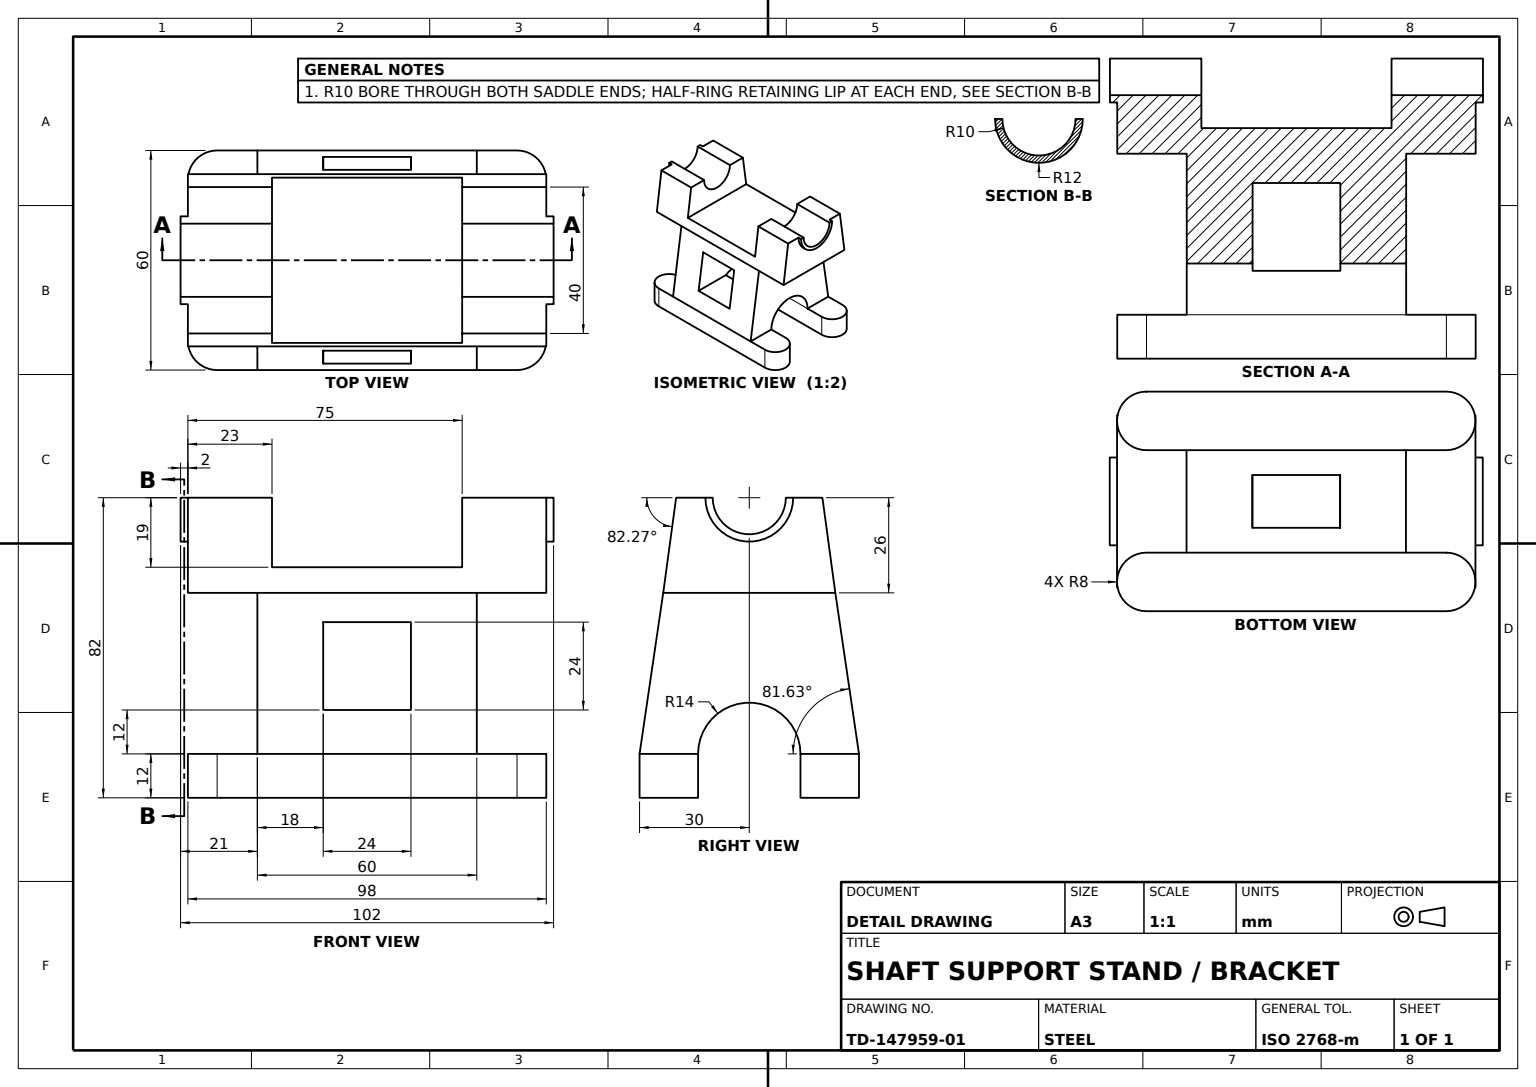
from build123d import *

# Parameters (mm, degrees)
BASE_BODY_DEPTH         = 12
BASE_BODY_2_DEPTH       = 12
FOOT_BOSS_60_DEPTH      = 60
WINDOW_CUT_DEPTH        = 60
SADDLE_ENDS_98_DEPTH    = 98
SADDLE_CRADLE_CUT_DEPTH = 19
ARCH_RELIEF_CUT_DEPTH   = 93
RETAINING_START         = 2
RETAINING_LIP_A_DEPTH   = 2
RETAINING_LIP_B_DEPTH   = 2


with BuildPart() as part:
    # Base Body Sketch → Base Body (new body)
    with BuildSketch(Plane(origin=(0, 0, 0), x_dir=(1, 0, 0), z_dir=(0, 1, 0))):
        with BuildLine():
            Line((-41, -14), (41, -14))
            ThreePointArc((41, -14), (49, -22), (41, -30))
            Line((41, -30), (-41, -30))
            ThreePointArc((-41, -30), (-49, -22), (-41, -14))
        make_face()
    extrude(amount=BASE_BODY_DEPTH)



with BuildPart() as body_2:
    # Base Body Sketch → Base Body 2 (new body)
    with BuildSketch(Plane(origin=(0, 0, 0), x_dir=(1, 0, 0), z_dir=(0, 1, 0))):
        with BuildLine():
            Line((41, 30), (-41, 30))
            ThreePointArc((-41, 30), (-49, 22), (-41, 14))
            Line((-41, 14), (41, 14))
            ThreePointArc((41, 14), (49, 22), (41, 30))
        make_face()
    extrude(amount=BASE_BODY_2_DEPTH)


with BuildPart() as part_1:
    add(part.part)

    add(body_2.part)  # Foot Boss 60 merges body 2
    # Foot Boss Sketch → Foot Boss 60 (add)
    with BuildSketch(Plane(origin=(30, 0, 0), x_dir=(0, 0, -1), z_dir=(1, 0, 0))):
        with BuildLine():
            Line((-14, 12), (-30, 12))
            Line((-30, 12), (-30, 56))
            Line((-30, 56), (30, 56))
            Line((30, 56), (30, 12))
            Line((30, 12), (14, 12))
            ThreePointArc((14, 12), (0, 26), (-14, 12))
        make_face()
    extrude(amount=-FOOT_BOSS_60_DEPTH)

    # Window Cut Sketch → Window Cut (cut)
    with BuildSketch(Plane(origin=(30, 0, 0), x_dir=(0, 0, -1), z_dir=(1, 0, 0))):
        Polygon((-23.08335547, 59.033182801), (-30, 12), (-33.835274918, 12), (-33.835274918, 59.033182801), align=None)
        Polygon((23.08335547, 59.033182801), (30, 12), (40.995792327, 12), (40.995792327, 59.033182801), align=None)
    extrude(amount=-WINDOW_CUT_DEPTH, mode=Mode.SUBTRACT)

    # Saddle Ends Sketch → Saddle Ends 98 (add)
    with BuildSketch(Plane(origin=(49, 0, 0), x_dir=(0, 0, -1), z_dir=(1, 0, 0))):
        with BuildLine():
            Line((10, 82), (20, 82))
            Line((20, 82), (23.529411765, 56))
            Line((23.529411765, 56), (-23.529411765, 56))
            Line((-23.529411765, 56), (-20, 82))
            Line((-20, 82), (-10, 82))
            ThreePointArc((-10, 82), (0, 72), (10, 82))
        make_face()
    extrude(amount=-SADDLE_ENDS_98_DEPTH)

    # Saddle Cradle Cut Sketch → Saddle Cradle Cut (cut)
    with BuildSketch(Plane(origin=(0, 82, 0), x_dir=(1, 0, 0), z_dir=(0, 1, 0))):
        Polygon((26, 0), (26, -36.490977082), (-26, -36.490977082), (-26, 35.721826881), (26, 35.721826881), align=None)
    extrude(amount=-SADDLE_CRADLE_CUT_DEPTH, mode=Mode.SUBTRACT)

    # Arch Relief Cut Sketch → Arch Relief Cut (cut)
    with BuildSketch(Plane(origin=(0, 0, -30), x_dir=(-1, 0, 0), z_dir=(0, 0, -1))):
        Polygon((0, 24), (12, 24), (12, 48), (-12, 48), (-12, 24), align=None)
    extrude(amount=-ARCH_RELIEF_CUT_DEPTH, mode=Mode.SUBTRACT)

    # Retaining Lip A Sketch → Retaining Lip A (add)
    with BuildSketch(Plane(origin=(49, 0, 0), x_dir=(0, 0, -1), z_dir=(1, 0, 0)).offset(RETAINING_START)):
        with BuildLine():
            Line((-12, 82), (-10, 82))
            ThreePointArc((-10, 82), (0, 72), (10, 82))
            Line((10, 82), (12, 82))
            ThreePointArc((12, 82), (0, 70), (-12, 82))
        make_face()
    extrude(amount=-RETAINING_LIP_A_DEPTH)

    # Retaining Lip B Sketch → Retaining Lip B (add)
    with BuildSketch(Plane.ZY.offset(49)):
        with BuildLine():
            Line((10, 82), (12, 82))
            ThreePointArc((12, 82), (0, 70), (-12, 82))
            Line((-12, 82), (-10, 82))
            ThreePointArc((-10, 82), (0, 72), (10, 82))
        make_face()
    extrude(amount=RETAINING_LIP_B_DEPTH)


solid = part_1.part
